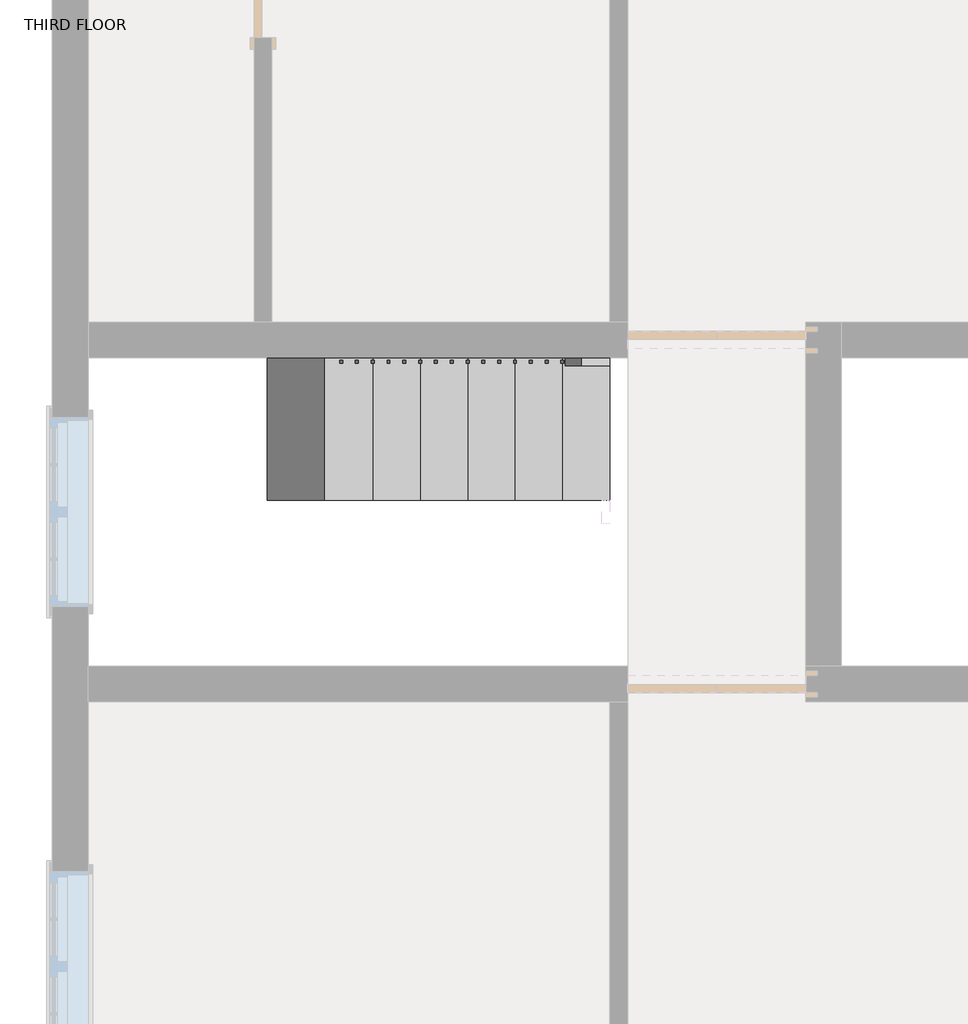
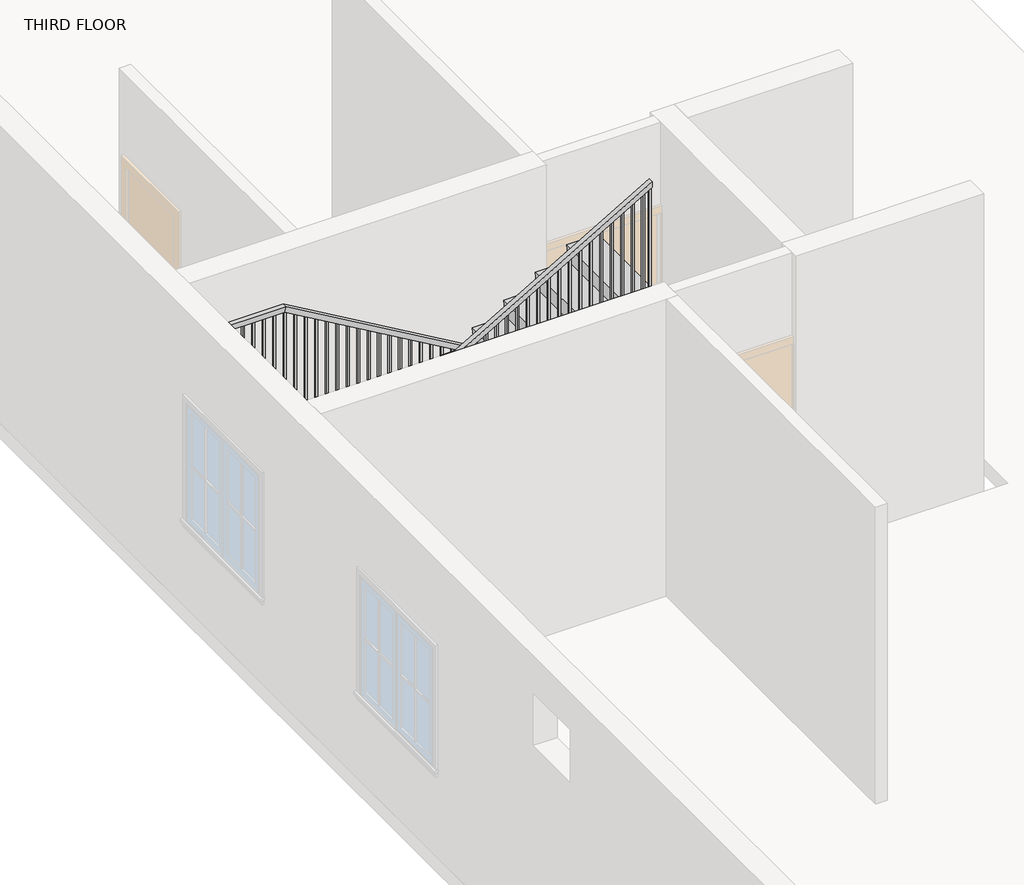
# One storey, part 3 of 4: 1 railing, 1 stair flight.
"""IFC4 building model written with IfcOpenShell, lengths in millimetres."""

from ifc_helpers import new_model, si_unit, frame, origin, place, context, project, spatial, polyline, outline, extrude, faceted_brep, element, save

model = new_model("IFC4")

# Units and contexts
model_context = context("Model", 3, world=origin())
ifc_project = project(units=[si_unit("LENGTHUNIT", "METRE", prefix="MILLI")], contexts=[model_context])

# Site, building, storey
site = spatial("IfcSite", under=ifc_project)
building = spatial("IfcBuilding", under=site)
storey = spatial("IfcBuildingStorey", under=building, Name="THIRD FLOOR", Elevation=9601.2)

# Railing
placement = place(None, origin())
element("IfcRailing", 1, ObjectType="Handrail - Rectangular", at=placement, inside=storey, context=model_context, shape_type="SolidModel", body=[
    faceted_brep([(-2776.8289041, 1499.0153263, 10693.4), (-2776.8289041, 1499.0153263, 10634.5886538), (-2776.8289041, 1549.8153263, 10634.5886538), (-2776.8289041, 1549.8153263, 10693.4), (-5215.2289041, 1499.0153263, 12115.8), (-5228.9626405, 1499.0153263, 12065.0), (-5228.9626405, 1549.8153263, 12065.0), (-5215.2289041, 1549.8153263, 12115.8), (-6078.8289041, 1499.0153263, 12115.8), (-6078.8289041, 1499.0153263, 12065.0), (-6129.6289041, 1549.8153263, 12065.0), (-6129.6289041, 1549.8153263, 12115.8), (-6078.8289041, -380.5846737, 12115.8), (-6078.8289041, -380.5846737, 12065.0), (-6129.6289041, -431.3846737, 12065.0), (-6129.6289041, -431.3846737, 12115.8), (-5520.0289041, -380.5846737, 12115.8), (-5506.2951677, -380.5846737, 12065.0), (-5506.2951677, -431.3846737, 12065.0), (-5520.0289041, -431.3846737, 12115.8), (-2776.8289041, -380.5846737, 13716.0), (-2776.8289041, -431.3846737, 13716.0), (-2776.8289041, -431.3846737, 13657.1886538), (-2776.8289041, -380.5846737, 13657.1886538)], [[[0, 1, 2, 3]], [[1, 0, 4, 5]], [[2, 1, 5, 6]], [[3, 2, 6, 7]], [[0, 3, 7, 4]], [[5, 4, 8, 9]], [[6, 5, 9, 10]], [[7, 6, 10, 11]], [[4, 7, 11, 8]], [[9, 8, 12, 13]], [[10, 9, 13, 14]], [[11, 10, 14, 15]], [[8, 11, 15, 12]], [[13, 12, 16, 17]], [[14, 13, 17, 18]], [[15, 14, 18, 19]], [[12, 15, 19, 16]], [[20, 21, 22, 23]], [[17, 16, 20, 23]], [[18, 17, 23, 22]], [[19, 18, 22, 21]], [[16, 19, 21, 20]]]),
    extrude(outline(polyline([(13618.2949038, -2843.5039041), (13607.1824038, -2862.5539041), (12623.8, -2862.5539041), (12623.8, -2843.5039041), (13618.2949038, -2843.5039041)])), frame((0.0, -415.5096737, 0.0), z_axis=(0.0, 1.0, 0.0), x_axis=(0.0, 0.0, 1.0)), (0.0, 0.0, 1.0), 19.05),
    extrude(outline(polyline([(13559.0282371, -2945.1039041), (13547.9157371, -2964.1539041), (12623.8, -2964.1539041), (12623.8, -2945.1039041), (13559.0282371, -2945.1039041)])), frame((0.0, -415.5096737, 0.0), z_axis=(0.0, 1.0, 0.0), x_axis=(0.0, 0.0, 1.0)), (0.0, 0.0, 1.0), 19.05),
    extrude(outline(polyline([(13499.7615704, -3046.7039041), (13488.6490704, -3065.7539041), (12623.8, -3065.7539041), (12623.8, -3046.7039041), (13499.7615704, -3046.7039041)])), frame((0.0, -415.5096737, 0.0), z_axis=(0.0, 1.0, 0.0), x_axis=(0.0, 0.0, 1.0)), (0.0, 0.0, 1.0), 19.05),
    extrude(outline(polyline([(13440.4949038, -3148.3039041), (13429.3824038, -3167.3539041), (12446.0, -3167.3539041), (12446.0, -3148.3039041), (13440.4949038, -3148.3039041)])), frame((0.0, -415.5096737, 0.0), z_axis=(0.0, 1.0, 0.0), x_axis=(0.0, 0.0, 1.0)), (0.0, 0.0, 1.0), 19.05),
    extrude(outline(polyline([(13381.2282371, -3249.9039041), (13370.1157371, -3268.9539041), (12446.0, -3268.9539041), (12446.0, -3249.9039041), (13381.2282371, -3249.9039041)])), frame((0.0, -415.5096737, 0.0), z_axis=(0.0, 1.0, 0.0), x_axis=(0.0, 0.0, 1.0)), (0.0, 0.0, 1.0), 19.05),
    extrude(outline(polyline([(13321.9615704, -3351.5039041), (13310.8490704, -3370.5539041), (12446.0, -3370.5539041), (12446.0, -3351.5039041), (13321.9615704, -3351.5039041)])), frame((0.0, -415.5096737, 0.0), z_axis=(0.0, 1.0, 0.0), x_axis=(0.0, 0.0, 1.0)), (0.0, 0.0, 1.0), 19.05),
    extrude(outline(polyline([(13262.6949038, -3453.1039041), (13251.5824038, -3472.1539041), (12268.2, -3472.1539041), (12268.2, -3453.1039041), (13262.6949038, -3453.1039041)])), frame((0.0, -415.5096737, 0.0), z_axis=(0.0, 1.0, 0.0), x_axis=(0.0, 0.0, 1.0)), (0.0, 0.0, 1.0), 19.05),
    extrude(outline(polyline([(13203.4282371, -3554.7039041), (13192.3157371, -3573.7539041), (12268.2, -3573.7539041), (12268.2, -3554.7039041), (13203.4282371, -3554.7039041)])), frame((0.0, -415.5096737, 0.0), z_axis=(0.0, 1.0, 0.0), x_axis=(0.0, 0.0, 1.0)), (0.0, 0.0, 1.0), 19.05),
    extrude(outline(polyline([(13144.1615704, -3656.3039041), (13133.0490704, -3675.3539041), (12268.2, -3675.3539041), (12268.2, -3656.3039041), (13144.1615704, -3656.3039041)])), frame((0.0, -415.5096737, 0.0), z_axis=(0.0, 1.0, 0.0), x_axis=(0.0, 0.0, 1.0)), (0.0, 0.0, 1.0), 19.05),
    extrude(outline(polyline([(13084.8949038, -3757.9039041), (13073.7824038, -3776.9539041), (12090.4, -3776.9539041), (12090.4, -3757.9039041), (13084.8949038, -3757.9039041)])), frame((0.0, -415.5096737, 0.0), z_axis=(0.0, 1.0, 0.0), x_axis=(0.0, 0.0, 1.0)), (0.0, 0.0, 1.0), 19.05),
    extrude(outline(polyline([(13025.6282371, -3859.5039041), (13014.5157371, -3878.5539041), (12090.4, -3878.5539041), (12090.4, -3859.5039041), (13025.6282371, -3859.5039041)])), frame((0.0, -415.5096737, 0.0), z_axis=(0.0, 1.0, 0.0), x_axis=(0.0, 0.0, 1.0)), (0.0, 0.0, 1.0), 19.05),
    extrude(outline(polyline([(12966.3615704, -3961.1039041), (12955.2490704, -3980.1539041), (12090.4, -3980.1539041), (12090.4, -3961.1039041), (12966.3615704, -3961.1039041)])), frame((0.0, -415.5096737, 0.0), z_axis=(0.0, 1.0, 0.0), x_axis=(0.0, 0.0, 1.0)), (0.0, 0.0, 1.0), 19.05),
    extrude(outline(polyline([(12907.0949038, -4062.7039041), (12895.9824038, -4081.7539041), (11912.6, -4081.7539041), (11912.6, -4062.7039041), (12907.0949038, -4062.7039041)])), frame((0.0, -415.5096737, 0.0), z_axis=(0.0, 1.0, 0.0), x_axis=(0.0, 0.0, 1.0)), (0.0, 0.0, 1.0), 19.05),
    extrude(outline(polyline([(12847.8282371, -4164.3039041), (12836.7157371, -4183.3539041), (11912.6, -4183.3539041), (11912.6, -4164.3039041), (12847.8282371, -4164.3039041)])), frame((0.0, -415.5096737, 0.0), z_axis=(0.0, 1.0, 0.0), x_axis=(0.0, 0.0, 1.0)), (0.0, 0.0, 1.0), 19.05),
    extrude(outline(polyline([(12788.5615704, -4265.9039041), (12777.4490704, -4284.9539041), (11912.6, -4284.9539041), (11912.6, -4265.9039041), (12788.5615704, -4265.9039041)])), frame((0.0, -415.5096737, 0.0), z_axis=(0.0, 1.0, 0.0), x_axis=(0.0, 0.0, 1.0)), (0.0, 0.0, 1.0), 19.05),
    extrude(outline(polyline([(12729.2949038, -4367.5039041), (12718.1824038, -4386.5539041), (11734.8, -4386.5539041), (11734.8, -4367.5039041), (12729.2949038, -4367.5039041)])), frame((0.0, -415.5096737, 0.0), z_axis=(0.0, 1.0, 0.0), x_axis=(0.0, 0.0, 1.0)), (0.0, 0.0, 1.0), 19.05),
    extrude(outline(polyline([(12670.0282371, -4469.1039041), (12658.9157371, -4488.1539041), (11734.8, -4488.1539041), (11734.8, -4469.1039041), (12670.0282371, -4469.1039041)])), frame((0.0, -415.5096737, 0.0), z_axis=(0.0, 1.0, 0.0), x_axis=(0.0, 0.0, 1.0)), (0.0, 0.0, 1.0), 19.05),
    extrude(outline(polyline([(12610.7615704, -4570.7039041), (12599.6490704, -4589.7539041), (11734.8, -4589.7539041), (11734.8, -4570.7039041), (12610.7615704, -4570.7039041)])), frame((0.0, -415.5096737, 0.0), z_axis=(0.0, 1.0, 0.0), x_axis=(0.0, 0.0, 1.0)), (0.0, 0.0, 1.0), 19.05),
    extrude(outline(polyline([(12551.4949038, -4672.3039041), (12540.3824038, -4691.3539041), (11557.0, -4691.3539041), (11557.0, -4672.3039041), (12551.4949038, -4672.3039041)])), frame((0.0, -415.5096737, 0.0), z_axis=(0.0, 1.0, 0.0), x_axis=(0.0, 0.0, 1.0)), (0.0, 0.0, 1.0), 19.05),
    extrude(outline(polyline([(12492.2282371, -4773.9039041), (12481.1157371, -4792.9539041), (11557.0, -4792.9539041), (11557.0, -4773.9039041), (12492.2282371, -4773.9039041)])), frame((0.0, -415.5096737, 0.0), z_axis=(0.0, 1.0, 0.0), x_axis=(0.0, 0.0, 1.0)), (0.0, 0.0, 1.0), 19.05),
    extrude(outline(polyline([(12432.9615704, -4875.5039041), (12421.8490704, -4894.5539041), (11557.0, -4894.5539041), (11557.0, -4875.5039041), (12432.9615704, -4875.5039041)])), frame((0.0, -415.5096737, 0.0), z_axis=(0.0, 1.0, 0.0), x_axis=(0.0, 0.0, 1.0)), (0.0, 0.0, 1.0), 19.05),
    extrude(outline(polyline([(12373.6949038, -4977.1039041), (12362.5824038, -4996.1539041), (11379.2, -4996.1539041), (11379.2, -4977.1039041), (12373.6949038, -4977.1039041)])), frame((0.0, -415.5096737, 0.0), z_axis=(0.0, 1.0, 0.0), x_axis=(0.0, 0.0, 1.0)), (0.0, 0.0, 1.0), 19.05),
    extrude(outline(polyline([(12314.4282371, -5078.7039041), (12303.3157371, -5097.7539041), (11379.2, -5097.7539041), (11379.2, -5078.7039041), (12314.4282371, -5078.7039041)])), frame((0.0, -415.5096737, 0.0), z_axis=(0.0, 1.0, 0.0), x_axis=(0.0, 0.0, 1.0)), (0.0, 0.0, 1.0), 19.05),
    extrude(outline(polyline([(12255.1615704, -5180.3039041), (12244.0490704, -5199.3539041), (11379.2, -5199.3539041), (11379.2, -5180.3039041), (12255.1615704, -5180.3039041)])), frame((0.0, -415.5096737, 0.0), z_axis=(0.0, 1.0, 0.0), x_axis=(0.0, 0.0, 1.0)), (0.0, 0.0, 1.0), 19.05),
    extrude(outline(polyline([(12195.8949038, -5281.9039041), (12184.7824038, -5300.9539041), (11201.4, -5300.9539041), (11201.4, -5281.9039041), (12195.8949038, -5281.9039041)])), frame((0.0, -415.5096737, 0.0), z_axis=(0.0, 1.0, 0.0), x_axis=(0.0, 0.0, 1.0)), (0.0, 0.0, 1.0), 19.05),
    extrude(outline(polyline([(12136.6282371, -5383.5039041), (12125.5157371, -5402.5539041), (11201.4, -5402.5539041), (11201.4, -5383.5039041), (12136.6282371, -5383.5039041)])), frame((0.0, -415.5096737, 0.0), z_axis=(0.0, 1.0, 0.0), x_axis=(0.0, 0.0, 1.0)), (0.0, 0.0, 1.0), 19.05),
    extrude(outline(polyline([(12077.3615704, -5485.1039041), (12066.2490704, -5504.1539041), (11201.4, -5504.1539041), (11201.4, -5485.1039041), (12077.3615704, -5485.1039041)])), frame((0.0, -415.5096737, 0.0), z_axis=(0.0, 1.0, 0.0), x_axis=(0.0, 0.0, 1.0)), (0.0, 0.0, 1.0), 19.05),
    extrude(outline(polyline([(-5605.7539041, -415.5096737), (-5605.7539041, -396.4596737), (-5586.7039041, -396.4596737), (-5586.7039041, -415.5096737), (-5605.7539041, -415.5096737)])), frame((0.0, 0.0, 11201.4), z_axis=(0.0, 0.0, 1.0), x_axis=(1.0, 0.0, 0.0)), (0.0, 0.0, 1.0), 863.6),
    extrude(outline(polyline([(-5707.3539041, -415.5096737), (-5707.3539041, -396.4596737), (-5688.3039041, -396.4596737), (-5688.3039041, -415.5096737), (-5707.3539041, -415.5096737)])), frame((0.0, 0.0, 11201.4), z_axis=(0.0, 0.0, 1.0), x_axis=(1.0, 0.0, 0.0)), (0.0, 0.0, 1.0), 863.6),
    extrude(outline(polyline([(-5808.9539041, -415.5096737), (-5808.9539041, -396.4596737), (-5789.9039041, -396.4596737), (-5789.9039041, -415.5096737), (-5808.9539041, -415.5096737)])), frame((0.0, 0.0, 11201.4), z_axis=(0.0, 0.0, 1.0), x_axis=(1.0, 0.0, 0.0)), (0.0, 0.0, 1.0), 863.6),
    extrude(outline(polyline([(-5910.5539041, -415.5096737), (-5910.5539041, -396.4596737), (-5891.5039041, -396.4596737), (-5891.5039041, -415.5096737), (-5910.5539041, -415.5096737)])), frame((0.0, 0.0, 11201.4), z_axis=(0.0, 0.0, 1.0), x_axis=(1.0, 0.0, 0.0)), (0.0, 0.0, 1.0), 863.6),
    extrude(outline(polyline([(-6012.1539041, -415.5096737), (-6012.1539041, -396.4596737), (-5993.1039041, -396.4596737), (-5993.1039041, -415.5096737), (-6012.1539041, -415.5096737)])), frame((0.0, 0.0, 11201.4), z_axis=(0.0, 0.0, 1.0), x_axis=(1.0, 0.0, 0.0)), (0.0, 0.0, 1.0), 863.6),
    extrude(outline(polyline([(-6113.7539041, -294.8596737), (-6094.7039041, -294.8596737), (-6094.7039041, -313.9096737), (-6113.7539041, -313.9096737), (-6113.7539041, -294.8596737)])), frame((0.0, 0.0, 11201.4), z_axis=(0.0, 0.0, 1.0), x_axis=(1.0, 0.0, 0.0)), (0.0, 0.0, 1.0), 863.6),
    extrude(outline(polyline([(-6113.7539041, -193.2596737), (-6094.7039041, -193.2596737), (-6094.7039041, -212.3096737), (-6113.7539041, -212.3096737), (-6113.7539041, -193.2596737)])), frame((0.0, 0.0, 11201.4), z_axis=(0.0, 0.0, 1.0), x_axis=(1.0, 0.0, 0.0)), (0.0, 0.0, 1.0), 863.6),
    extrude(outline(polyline([(-6113.7539041, -91.6596737), (-6094.7039041, -91.6596737), (-6094.7039041, -110.7096737), (-6113.7539041, -110.7096737), (-6113.7539041, -91.6596737)])), frame((0.0, 0.0, 11201.4), z_axis=(0.0, 0.0, 1.0), x_axis=(1.0, 0.0, 0.0)), (0.0, 0.0, 1.0), 863.6),
    extrude(outline(polyline([(-6113.7539041, 9.9403263), (-6094.7039041, 9.9403263), (-6094.7039041, -9.1096737), (-6113.7539041, -9.1096737), (-6113.7539041, 9.9403263)])), frame((0.0, 0.0, 11201.4), z_axis=(0.0, 0.0, 1.0), x_axis=(1.0, 0.0, 0.0)), (0.0, 0.0, 1.0), 863.6),
    extrude(outline(polyline([(-6113.7539041, 111.5403263), (-6094.7039041, 111.5403263), (-6094.7039041, 92.4903263), (-6113.7539041, 92.4903263), (-6113.7539041, 111.5403263)])), frame((0.0, 0.0, 11201.4), z_axis=(0.0, 0.0, 1.0), x_axis=(1.0, 0.0, 0.0)), (0.0, 0.0, 1.0), 863.6),
    extrude(outline(polyline([(-6113.7539041, 213.1403263), (-6094.7039041, 213.1403263), (-6094.7039041, 194.0903263), (-6113.7539041, 194.0903263), (-6113.7539041, 213.1403263)])), frame((0.0, 0.0, 11201.4), z_axis=(0.0, 0.0, 1.0), x_axis=(1.0, 0.0, 0.0)), (0.0, 0.0, 1.0), 863.6),
    extrude(outline(polyline([(-6113.7539041, 314.7403263), (-6094.7039041, 314.7403263), (-6094.7039041, 295.6903263), (-6113.7539041, 295.6903263), (-6113.7539041, 314.7403263)])), frame((0.0, 0.0, 11201.4), z_axis=(0.0, 0.0, 1.0), x_axis=(1.0, 0.0, 0.0)), (0.0, 0.0, 1.0), 863.6),
    extrude(outline(polyline([(-6113.7539041, 416.3403263), (-6094.7039041, 416.3403263), (-6094.7039041, 397.2903263), (-6113.7539041, 397.2903263), (-6113.7539041, 416.3403263)])), frame((0.0, 0.0, 11201.4), z_axis=(0.0, 0.0, 1.0), x_axis=(1.0, 0.0, 0.0)), (0.0, 0.0, 1.0), 863.6),
    extrude(outline(polyline([(-6113.7539041, 517.9403263), (-6094.7039041, 517.9403263), (-6094.7039041, 498.8903263), (-6113.7539041, 498.8903263), (-6113.7539041, 517.9403263)])), frame((0.0, 0.0, 11201.4), z_axis=(0.0, 0.0, 1.0), x_axis=(1.0, 0.0, 0.0)), (0.0, 0.0, 1.0), 863.6),
    extrude(outline(polyline([(-6113.7539041, 619.5403263), (-6094.7039041, 619.5403263), (-6094.7039041, 600.4903263), (-6113.7539041, 600.4903263), (-6113.7539041, 619.5403263)])), frame((0.0, 0.0, 11201.4), z_axis=(0.0, 0.0, 1.0), x_axis=(1.0, 0.0, 0.0)), (0.0, 0.0, 1.0), 863.6),
    extrude(outline(polyline([(-6113.7539041, 721.1403263), (-6094.7039041, 721.1403263), (-6094.7039041, 702.0903263), (-6113.7539041, 702.0903263), (-6113.7539041, 721.1403263)])), frame((0.0, 0.0, 11201.4), z_axis=(0.0, 0.0, 1.0), x_axis=(1.0, 0.0, 0.0)), (0.0, 0.0, 1.0), 863.6),
    extrude(outline(polyline([(-6113.7539041, 822.7403263), (-6094.7039041, 822.7403263), (-6094.7039041, 803.6903263), (-6113.7539041, 803.6903263), (-6113.7539041, 822.7403263)])), frame((0.0, 0.0, 11201.4), z_axis=(0.0, 0.0, 1.0), x_axis=(1.0, 0.0, 0.0)), (0.0, 0.0, 1.0), 863.6),
    extrude(outline(polyline([(-6113.7539041, 924.3403263), (-6094.7039041, 924.3403263), (-6094.7039041, 905.2903263), (-6113.7539041, 905.2903263), (-6113.7539041, 924.3403263)])), frame((0.0, 0.0, 11201.4), z_axis=(0.0, 0.0, 1.0), x_axis=(1.0, 0.0, 0.0)), (0.0, 0.0, 1.0), 863.6),
    extrude(outline(polyline([(-6113.7539041, 1025.9403263), (-6094.7039041, 1025.9403263), (-6094.7039041, 1006.8903263), (-6113.7539041, 1006.8903263), (-6113.7539041, 1025.9403263)])), frame((0.0, 0.0, 11201.4), z_axis=(0.0, 0.0, 1.0), x_axis=(1.0, 0.0, 0.0)), (0.0, 0.0, 1.0), 863.6),
    extrude(outline(polyline([(-6113.7539041, 1127.5403263), (-6094.7039041, 1127.5403263), (-6094.7039041, 1108.4903263), (-6113.7539041, 1108.4903263), (-6113.7539041, 1127.5403263)])), frame((0.0, 0.0, 11201.4), z_axis=(0.0, 0.0, 1.0), x_axis=(1.0, 0.0, 0.0)), (0.0, 0.0, 1.0), 863.6),
    extrude(outline(polyline([(-6113.7539041, 1229.1403263), (-6094.7039041, 1229.1403263), (-6094.7039041, 1210.0903263), (-6113.7539041, 1210.0903263), (-6113.7539041, 1229.1403263)])), frame((0.0, 0.0, 11201.4), z_axis=(0.0, 0.0, 1.0), x_axis=(1.0, 0.0, 0.0)), (0.0, 0.0, 1.0), 863.6),
    extrude(outline(polyline([(-6113.7539041, 1330.7403263), (-6094.7039041, 1330.7403263), (-6094.7039041, 1311.6903263), (-6113.7539041, 1311.6903263), (-6113.7539041, 1330.7403263)])), frame((0.0, 0.0, 11201.4), z_axis=(0.0, 0.0, 1.0), x_axis=(1.0, 0.0, 0.0)), (0.0, 0.0, 1.0), 863.6),
    extrude(outline(polyline([(-6113.7539041, 1432.3403263), (-6094.7039041, 1432.3403263), (-6094.7039041, 1413.2903263), (-6113.7539041, 1413.2903263), (-6113.7539041, 1432.3403263)])), frame((0.0, 0.0, 11201.4), z_axis=(0.0, 0.0, 1.0), x_axis=(1.0, 0.0, 0.0)), (0.0, 0.0, 1.0), 863.6),
    extrude(outline(polyline([(-6018.5039041, 1533.9403263), (-6018.5039041, 1514.8903263), (-6037.5539041, 1514.8903263), (-6037.5539041, 1533.9403263), (-6018.5039041, 1533.9403263)])), frame((0.0, 0.0, 11201.4), z_axis=(0.0, 0.0, 1.0), x_axis=(1.0, 0.0, 0.0)), (0.0, 0.0, 1.0), 863.6),
    extrude(outline(polyline([(-5916.9039041, 1533.9403263), (-5916.9039041, 1514.8903263), (-5935.9539041, 1514.8903263), (-5935.9539041, 1533.9403263), (-5916.9039041, 1533.9403263)])), frame((0.0, 0.0, 11201.4), z_axis=(0.0, 0.0, 1.0), x_axis=(1.0, 0.0, 0.0)), (0.0, 0.0, 1.0), 863.6),
    extrude(outline(polyline([(-5815.3039041, 1533.9403263), (-5815.3039041, 1514.8903263), (-5834.3539041, 1514.8903263), (-5834.3539041, 1533.9403263), (-5815.3039041, 1533.9403263)])), frame((0.0, 0.0, 11201.4), z_axis=(0.0, 0.0, 1.0), x_axis=(1.0, 0.0, 0.0)), (0.0, 0.0, 1.0), 863.6),
    extrude(outline(polyline([(-5713.7039041, 1533.9403263), (-5713.7039041, 1514.8903263), (-5732.7539041, 1514.8903263), (-5732.7539041, 1533.9403263), (-5713.7039041, 1533.9403263)])), frame((0.0, 0.0, 11201.4), z_axis=(0.0, 0.0, 1.0), x_axis=(1.0, 0.0, 0.0)), (0.0, 0.0, 1.0), 863.6),
    extrude(outline(polyline([(-5612.1039041, 1533.9403263), (-5612.1039041, 1514.8903263), (-5631.1539041, 1514.8903263), (-5631.1539041, 1533.9403263), (-5612.1039041, 1533.9403263)])), frame((0.0, 0.0, 11201.4), z_axis=(0.0, 0.0, 1.0), x_axis=(1.0, 0.0, 0.0)), (0.0, 0.0, 1.0), 863.6),
    extrude(outline(polyline([(-5510.5039041, 1533.9403263), (-5510.5039041, 1514.8903263), (-5529.5539041, 1514.8903263), (-5529.5539041, 1533.9403263), (-5510.5039041, 1533.9403263)])), frame((0.0, 0.0, 11201.4), z_axis=(0.0, 0.0, 1.0), x_axis=(1.0, 0.0, 0.0)), (0.0, 0.0, 1.0), 863.6),
    extrude(outline(polyline([(-5408.9039041, 1533.9403263), (-5408.9039041, 1514.8903263), (-5427.9539041, 1514.8903263), (-5427.9539041, 1533.9403263), (-5408.9039041, 1533.9403263)])), frame((0.0, 0.0, 11201.4), z_axis=(0.0, 0.0, 1.0), x_axis=(1.0, 0.0, 0.0)), (0.0, 0.0, 1.0), 863.6),
    extrude(outline(polyline([(-5307.3039041, 1533.9403263), (-5307.3039041, 1514.8903263), (-5326.3539041, 1514.8903263), (-5326.3539041, 1533.9403263), (-5307.3039041, 1533.9403263)])), frame((0.0, 0.0, 11201.4), z_axis=(0.0, 0.0, 1.0), x_axis=(1.0, 0.0, 0.0)), (0.0, 0.0, 1.0), 863.6),
    extrude(outline(polyline([(12051.4324038, -5205.7039041), (12062.5449038, -5224.7539041), (11201.4, -5224.7539041), (11201.4, -5205.7039041), (12051.4324038, -5205.7039041)])), frame((0.0, 1514.8903263, 0.0), z_axis=(0.0, 1.0, 0.0), x_axis=(0.0, 0.0, 1.0)), (0.0, 0.0, 1.0), 19.05),
    extrude(outline(polyline([(11992.1657371, -5104.1039041), (12003.2782371, -5123.1539041), (11023.6, -5123.1539041), (11023.6, -5104.1039041), (11992.1657371, -5104.1039041)])), frame((0.0, 1514.8903263, 0.0), z_axis=(0.0, 1.0, 0.0), x_axis=(0.0, 0.0, 1.0)), (0.0, 0.0, 1.0), 19.05),
    extrude(outline(polyline([(11932.8990704, -5002.5039041), (11944.0115704, -5021.5539041), (11023.6, -5021.5539041), (11023.6, -5002.5039041), (11932.8990704, -5002.5039041)])), frame((0.0, 1514.8903263, 0.0), z_axis=(0.0, 1.0, 0.0), x_axis=(0.0, 0.0, 1.0)), (0.0, 0.0, 1.0), 19.05),
    extrude(outline(polyline([(11873.6324038, -4900.9039041), (11884.7449038, -4919.9539041), (11023.6, -4919.9539041), (11023.6, -4900.9039041), (11873.6324038, -4900.9039041)])), frame((0.0, 1514.8903263, 0.0), z_axis=(0.0, 1.0, 0.0), x_axis=(0.0, 0.0, 1.0)), (0.0, 0.0, 1.0), 19.05),
    extrude(outline(polyline([(11814.3657371, -4799.3039041), (11825.4782371, -4818.3539041), (10845.8, -4818.3539041), (10845.8, -4799.3039041), (11814.3657371, -4799.3039041)])), frame((0.0, 1514.8903263, 0.0), z_axis=(0.0, 1.0, 0.0), x_axis=(0.0, 0.0, 1.0)), (0.0, 0.0, 1.0), 19.05),
    extrude(outline(polyline([(11755.0990704, -4697.7039041), (11766.2115704, -4716.7539041), (10845.8, -4716.7539041), (10845.8, -4697.7039041), (11755.0990704, -4697.7039041)])), frame((0.0, 1514.8903263, 0.0), z_axis=(0.0, 1.0, 0.0), x_axis=(0.0, 0.0, 1.0)), (0.0, 0.0, 1.0), 19.05),
    extrude(outline(polyline([(11695.8324038, -4596.1039041), (11706.9449038, -4615.1539041), (10845.8, -4615.1539041), (10845.8, -4596.1039041), (11695.8324038, -4596.1039041)])), frame((0.0, 1514.8903263, 0.0), z_axis=(0.0, 1.0, 0.0), x_axis=(0.0, 0.0, 1.0)), (0.0, 0.0, 1.0), 19.05),
    extrude(outline(polyline([(11636.5657371, -4494.5039041), (11647.6782371, -4513.5539041), (10668.0, -4513.5539041), (10668.0, -4494.5039041), (11636.5657371, -4494.5039041)])), frame((0.0, 1514.8903263, 0.0), z_axis=(0.0, 1.0, 0.0), x_axis=(0.0, 0.0, 1.0)), (0.0, 0.0, 1.0), 19.05),
    extrude(outline(polyline([(11577.2990704, -4392.9039041), (11588.4115704, -4411.9539041), (10668.0, -4411.9539041), (10668.0, -4392.9039041), (11577.2990704, -4392.9039041)])), frame((0.0, 1514.8903263, 0.0), z_axis=(0.0, 1.0, 0.0), x_axis=(0.0, 0.0, 1.0)), (0.0, 0.0, 1.0), 19.05),
    extrude(outline(polyline([(11518.0324038, -4291.3039041), (11529.1449038, -4310.3539041), (10668.0, -4310.3539041), (10668.0, -4291.3039041), (11518.0324038, -4291.3039041)])), frame((0.0, 1514.8903263, 0.0), z_axis=(0.0, 1.0, 0.0), x_axis=(0.0, 0.0, 1.0)), (0.0, 0.0, 1.0), 19.05),
    extrude(outline(polyline([(11458.7657371, -4189.7039041), (11469.8782371, -4208.7539041), (10490.2, -4208.7539041), (10490.2, -4189.7039041), (11458.7657371, -4189.7039041)])), frame((0.0, 1514.8903263, 0.0), z_axis=(0.0, 1.0, 0.0), x_axis=(0.0, 0.0, 1.0)), (0.0, 0.0, 1.0), 19.05),
    extrude(outline(polyline([(11399.4990704, -4088.1039041), (11410.6115704, -4107.1539041), (10490.2, -4107.1539041), (10490.2, -4088.1039041), (11399.4990704, -4088.1039041)])), frame((0.0, 1514.8903263, 0.0), z_axis=(0.0, 1.0, 0.0), x_axis=(0.0, 0.0, 1.0)), (0.0, 0.0, 1.0), 19.05),
    extrude(outline(polyline([(11340.2324038, -3986.5039041), (11351.3449038, -4005.5539041), (10490.2, -4005.5539041), (10490.2, -3986.5039041), (11340.2324038, -3986.5039041)])), frame((0.0, 1514.8903263, 0.0), z_axis=(0.0, 1.0, 0.0), x_axis=(0.0, 0.0, 1.0)), (0.0, 0.0, 1.0), 19.05),
    extrude(outline(polyline([(11280.9657371, -3884.9039041), (11292.0782371, -3903.9539041), (10312.4, -3903.9539041), (10312.4, -3884.9039041), (11280.9657371, -3884.9039041)])), frame((0.0, 1514.8903263, 0.0), z_axis=(0.0, 1.0, 0.0), x_axis=(0.0, 0.0, 1.0)), (0.0, 0.0, 1.0), 19.05),
    extrude(outline(polyline([(11221.6990704, -3783.3039041), (11232.8115704, -3802.3539041), (10312.4, -3802.3539041), (10312.4, -3783.3039041), (11221.6990704, -3783.3039041)])), frame((0.0, 1514.8903263, 0.0), z_axis=(0.0, 1.0, 0.0), x_axis=(0.0, 0.0, 1.0)), (0.0, 0.0, 1.0), 19.05),
    extrude(outline(polyline([(11162.4324038, -3681.7039041), (11173.5449038, -3700.7539041), (10312.4, -3700.7539041), (10312.4, -3681.7039041), (11162.4324038, -3681.7039041)])), frame((0.0, 1514.8903263, 0.0), z_axis=(0.0, 1.0, 0.0), x_axis=(0.0, 0.0, 1.0)), (0.0, 0.0, 1.0), 19.05),
    extrude(outline(polyline([(11103.1657371, -3580.1039041), (11114.2782371, -3599.1539041), (10134.6, -3599.1539041), (10134.6, -3580.1039041), (11103.1657371, -3580.1039041)])), frame((0.0, 1514.8903263, 0.0), z_axis=(0.0, 1.0, 0.0), x_axis=(0.0, 0.0, 1.0)), (0.0, 0.0, 1.0), 19.05),
    extrude(outline(polyline([(11043.8990704, -3478.5039041), (11055.0115704, -3497.5539041), (10134.6, -3497.5539041), (10134.6, -3478.5039041), (11043.8990704, -3478.5039041)])), frame((0.0, 1514.8903263, 0.0), z_axis=(0.0, 1.0, 0.0), x_axis=(0.0, 0.0, 1.0)), (0.0, 0.0, 1.0), 19.05),
    extrude(outline(polyline([(10984.6324038, -3376.9039041), (10995.7449038, -3395.9539041), (10134.6, -3395.9539041), (10134.6, -3376.9039041), (10984.6324038, -3376.9039041)])), frame((0.0, 1514.8903263, 0.0), z_axis=(0.0, 1.0, 0.0), x_axis=(0.0, 0.0, 1.0)), (0.0, 0.0, 1.0), 19.05),
    extrude(outline(polyline([(10925.3657371, -3275.3039041), (10936.4782371, -3294.3539041), (9956.8, -3294.3539041), (9956.8, -3275.3039041), (10925.3657371, -3275.3039041)])), frame((0.0, 1514.8903263, 0.0), z_axis=(0.0, 1.0, 0.0), x_axis=(0.0, 0.0, 1.0)), (0.0, 0.0, 1.0), 19.05),
    extrude(outline(polyline([(10866.0990704, -3173.7039041), (10877.2115704, -3192.7539041), (9956.8, -3192.7539041), (9956.8, -3173.7039041), (10866.0990704, -3173.7039041)])), frame((0.0, 1514.8903263, 0.0), z_axis=(0.0, 1.0, 0.0), x_axis=(0.0, 0.0, 1.0)), (0.0, 0.0, 1.0), 19.05),
    extrude(outline(polyline([(10806.8324038, -3072.1039041), (10817.9449038, -3091.1539041), (9956.8, -3091.1539041), (9956.8, -3072.1039041), (10806.8324038, -3072.1039041)])), frame((0.0, 1514.8903263, 0.0), z_axis=(0.0, 1.0, 0.0), x_axis=(0.0, 0.0, 1.0)), (0.0, 0.0, 1.0), 19.05),
    extrude(outline(polyline([(10747.5657371, -2970.5039041), (10758.6782371, -2989.5539041), (9779.0, -2989.5539041), (9779.0, -2970.5039041), (10747.5657371, -2970.5039041)])), frame((0.0, 1514.8903263, 0.0), z_axis=(0.0, 1.0, 0.0), x_axis=(0.0, 0.0, 1.0)), (0.0, 0.0, 1.0), 19.05),
    extrude(outline(polyline([(10688.2990704, -2868.9039041), (10699.4115704, -2887.9539041), (9779.0, -2887.9539041), (9779.0, -2868.9039041), (10688.2990704, -2868.9039041)])), frame((0.0, 1514.8903263, 0.0), z_axis=(0.0, 1.0, 0.0), x_axis=(0.0, 0.0, 1.0)), (0.0, 0.0, 1.0), 19.05),
    extrude(outline(polyline([(-6113.7539041, -396.4596737), (-6094.7039041, -396.4596737), (-6094.7039041, -415.5096737), (-6113.7539041, -415.5096737), (-6113.7539041, -396.4596737)])), frame((0.0, 0.0, 11201.4), z_axis=(0.0, 0.0, 1.0), x_axis=(1.0, 0.0, 0.0)), (0.0, 0.0, 1.0), 863.6),
    extrude(outline(polyline([(-6094.7039041, 1533.9403263), (-6094.7039041, 1514.8903263), (-6113.7539041, 1514.8903263), (-6113.7539041, 1533.9403263), (-6094.7039041, 1533.9403263)])), frame((0.0, 0.0, 11201.4), z_axis=(0.0, 0.0, 1.0), x_axis=(1.0, 0.0, 0.0)), (0.0, 0.0, 1.0), 863.6),
    extrude(outline(polyline([(13657.1886538, -2776.8289041), (13646.0761538, -2795.8789041), (12623.8, -2795.8789041), (12623.8, -2776.8289041), (13657.1886538, -2776.8289041)])), frame((0.0, -415.5096737, 0.0), z_axis=(0.0, 1.0, 0.0), x_axis=(0.0, 0.0, 1.0)), (0.0, 0.0, 1.0), 19.05),
    extrude(outline(polyline([(10634.5886538, -2776.8289041), (10645.7011538, -2795.8789041), (9779.0, -2795.8789041), (9779.0, -2776.8289041), (10634.5886538, -2776.8289041)])), frame((0.0, 1514.8903263, 0.0), z_axis=(0.0, 1.0, 0.0), x_axis=(0.0, 0.0, 1.0)), (0.0, 0.0, 1.0), 19.05),
])

# Stair flight
element("IfcStairFlight", 2, ObjectType="3/4\" Nosing", at=placement, inside=storey, context=model_context, shape_type="Brep", body=[
    faceted_brep([(-2776.8289041, 635.4153263, 9779.0), (-2776.8289041, 1549.8153263, 9779.0), (-3100.6789041, 1549.8153263, 9779.0), (-3100.6789041, 635.4153263, 9779.0), (-3100.6789041, 635.4153263, 9705.4858172), (-2921.9032174, 635.4153263, 9601.2), (-2795.8789041, 635.4153263, 9601.2), (-2795.8789041, 1549.8153263, 9601.2), (-2921.9032174, 1549.8153263, 9601.2), (-3100.6789041, 1549.8153263, 9705.4858172), (-3081.6289041, 635.4153263, 9956.8), (-3081.6289041, 1549.8153263, 9956.8), (-3405.4789041, 1549.8153263, 9956.8), (-3405.4789041, 635.4153263, 9956.8), (-3405.4789041, 635.4153263, 9883.2858172), (-3405.4789041, 1549.8153263, 9883.2858172), (-3386.4289041, 635.4153263, 10134.6), (-3386.4289041, 1549.8153263, 10134.6), (-3710.2789041, 1549.8153263, 10134.6), (-3710.2789041, 635.4153263, 10134.6), (-3710.2789041, 635.4153263, 10061.0858172), (-3710.2789041, 1549.8153263, 10061.0858172), (-3691.2289041, 635.4153263, 10312.4), (-3691.2289041, 1549.8153263, 10312.4), (-4015.0789041, 1549.8153263, 10312.4), (-4015.0789041, 635.4153263, 10312.4), (-4015.0789041, 635.4153263, 10238.8858172), (-4015.0789041, 1549.8153263, 10238.8858172), (-3996.0289041, 635.4153263, 10490.2), (-3996.0289041, 1549.8153263, 10490.2), (-4319.8789041, 1549.8153263, 10490.2), (-4319.8789041, 635.4153263, 10490.2), (-4300.8289041, 635.4153263, 10668.0), (-4624.6789041, 635.4153263, 10668.0), (-4605.6289041, 635.4153263, 10845.8), (-4929.4789041, 635.4153263, 10845.8), (-4910.4289041, 635.4153263, 11023.6), (-5234.2789041, 635.4153263, 11023.6), (-5222.0324755, 635.4153263, 11137.9), (-5556.2460745, 635.4153263, 11137.9), (-4319.8789041, 1549.8153263, 10416.6858172), (-4300.8289041, 1549.8153263, 10668.0), (-4624.6789041, 1549.8153263, 10668.0), (-4624.6789041, 1549.8153263, 10594.4858172), (-4605.6289041, 1549.8153263, 10845.8), (-4929.4789041, 1549.8153263, 10845.8), (-4929.4789041, 1549.8153263, 10772.2858172), (-4910.4289041, 1549.8153263, 11023.6), (-5234.2789041, 1549.8153263, 11023.6), (-5234.2789041, 1549.8153263, 10950.0858172), (-5070.1545907, 483.0153263, 11201.4), (-2776.8289041, 483.0153263, 11201.4), (-2776.8289041, 635.4153263, 11201.4), (-3836.3032174, 635.4153263, 11201.4), (-5215.2289041, 635.4153263, 11201.4), (-5215.2289041, 1549.8153263, 11201.4), (-5556.2460745, 1549.8153263, 11201.4), (-6129.6289041, 1549.8153263, 11201.4), (-6129.6289041, -431.3846737, 11201.4), (-5196.1789041, -431.3846737, 11201.4), (-5196.1789041, 483.0153263, 11201.4), (-5179.0117336, 483.0153263, 11137.9), (-2776.8289041, 483.0153263, 11137.9), (-2776.8289041, 635.4153263, 11137.9), (-3727.4460745, 635.4153263, 11137.9), (-5556.2460745, 1549.8153263, 11137.9), (-6129.6289041, 1549.8153263, 11137.9), (-6129.6289041, -431.3846737, 11137.9), (-5196.1789041, -431.3846737, 11137.9), (-5215.2289041, 483.0153263, 11379.2), (-5215.2289041, -431.3846737, 11379.2), (-5179.0117336, -431.3846737, 11379.2), (-4891.3789041, -431.3846737, 11379.2), (-4891.3789041, 483.0153263, 11379.2), (-4891.3789041, 483.0153263, 11305.6858172), (-5179.0117336, -431.3846737, 11137.9), (-4891.3789041, -431.3846737, 11305.6858172), (-4910.4289041, 483.0153263, 11557.0), (-4910.4289041, -431.3846737, 11557.0), (-4586.5789041, -431.3846737, 11557.0), (-4586.5789041, 483.0153263, 11557.0), (-4586.5789041, 483.0153263, 11483.4858172), (-4586.5789041, -431.3846737, 11483.4858172), (-4605.6289041, 483.0153263, 11734.8), (-4605.6289041, -431.3846737, 11734.8), (-4281.7789041, -431.3846737, 11734.8), (-4281.7789041, 483.0153263, 11734.8), (-4281.7789041, 483.0153263, 11671.3), (-4281.7789041, 483.0153263, 11661.2858172), (-4598.8253326, 483.0153263, 11671.3), (-4281.7789041, -431.3846737, 11661.2858172), (-4300.8289041, 483.0153263, 11912.6), (-4300.8289041, -431.3846737, 11912.6), (-3976.9789041, -431.3846737, 11912.6), (-3976.9789041, 483.0153263, 11912.6), (-3976.9789041, 483.0153263, 11839.0858172), (-4264.6117336, 483.0153263, 11671.3), (-3976.9789041, -431.3846737, 11839.0858172), (-3996.0289041, 483.0153263, 12090.4), (-3996.0289041, -431.3846737, 12090.4), (-3672.1789041, -431.3846737, 12090.4), (-3672.1789041, 483.0153263, 12090.4), (-3672.1789041, 483.0153263, 12016.8858172), (-3672.1789041, -431.3846737, 12016.8858172), (-3691.2289041, 483.0153263, 12268.2), (-3691.2289041, -431.3846737, 12268.2), (-3367.3789041, -431.3846737, 12268.2), (-3367.3789041, 483.0153263, 12268.2), (-3367.3789041, 483.0153263, 12194.6858172), (-3367.3789041, -431.3846737, 12194.6858172), (-3386.4289041, 483.0153263, 12446.0), (-3386.4289041, -431.3846737, 12446.0), (-3062.5789041, -431.3846737, 12446.0), (-3062.5789041, 483.0153263, 12446.0), (-3062.5789041, 483.0153263, 12372.4858172), (-3062.5789041, -431.3846737, 12372.4858172), (-3081.6289041, 483.0153263, 12623.8), (-3081.6289041, -431.3846737, 12623.8), (-2776.8289041, -431.3846737, 12623.8), (-2776.8289041, 483.0153263, 12623.8), (-2776.8289041, 483.0153263, 12539.1733172), (-2776.8289041, -431.3846737, 12539.1733172)], [[[0, 1, 2, 3]], [[0, 3, 4, 5, 6]], [[2, 1, 7, 8, 9]], [[10, 11, 12, 13]], [[10, 13, 14, 4, 3]], [[12, 11, 2, 9, 15]], [[16, 17, 18, 19]], [[16, 19, 20, 14, 13]], [[18, 17, 12, 15, 21]], [[22, 23, 24, 25]], [[22, 25, 26, 20, 19]], [[24, 23, 18, 21, 27]], [[28, 29, 30, 31]], [[26, 25, 28, 31, 32, 33, 34, 35, 36, 37, 38, 39]], [[30, 29, 24, 27, 40]], [[32, 41, 42, 33]], [[42, 41, 30, 40, 43]], [[34, 44, 45, 35]], [[45, 44, 42, 43, 46]], [[36, 47, 48, 37]], [[48, 47, 45, 46, 49]], [[50, 51, 52, 53, 54, 55, 56, 57, 58, 59, 60]], [[50, 61, 62, 51]], [[52, 51, 62, 63]], [[52, 63, 64, 38, 54, 53]], [[55, 48, 49, 65, 66, 57, 56]], [[58, 57, 66, 67]], [[59, 58, 67, 68]], [[69, 70, 71, 72, 73]], [[69, 73, 74, 50, 60]], [[70, 59, 68, 75, 76, 72, 71]], [[77, 78, 79, 80]], [[77, 80, 81, 74, 73]], [[79, 78, 72, 76, 82]], [[83, 84, 85, 86]], [[83, 86, 87, 88, 81, 80, 89]], [[85, 84, 79, 82, 90]], [[91, 92, 93, 94]], [[91, 94, 95, 96, 88, 87, 86]], [[93, 92, 85, 90, 97]], [[98, 99, 100, 101]], [[98, 101, 102, 95, 94]], [[100, 99, 93, 97, 103]], [[104, 105, 106, 107]], [[104, 107, 108, 102, 101]], [[106, 105, 100, 103, 109]], [[110, 111, 112, 113]], [[110, 113, 114, 108, 107]], [[112, 111, 106, 109, 115]], [[1, 0, 6, 7]], [[3, 2, 11, 10]], [[13, 12, 17, 16]], [[19, 18, 23, 22]], [[25, 24, 29, 28]], [[31, 30, 41, 32]], [[33, 42, 44, 34]], [[35, 45, 47, 36]], [[37, 48, 55, 54, 38]], [[60, 59, 70, 69]], [[73, 72, 78, 77]], [[80, 79, 84, 83, 89]], [[86, 85, 92, 91]], [[94, 93, 99, 98]], [[101, 100, 105, 104]], [[107, 106, 111, 110]], [[116, 117, 118, 119]], [[116, 119, 120, 114, 113]], [[118, 117, 112, 115, 121]], [[119, 118, 121, 120]], [[113, 112, 117, 116]], [[7, 6, 5, 8]], [[26, 39, 65, 49, 46, 43, 40, 27, 21, 15, 9, 8, 5, 4, 14, 20]], [[65, 39, 38, 64, 63, 62, 61, 75, 68, 67, 66]], [[75, 61, 50, 74, 81, 88, 96, 95, 102, 108, 114, 120, 121, 115, 109, 103, 97, 90, 82, 76]]]),
])

save(model, "model.ifc")

# Revit data of these elements
# Type "Handrail - Rectangular"
#   Assembly Code = "C2010400"
#   built-in parameter 1008612 = 0.0416667 (stored number, unit not read)
#   built-in parameter 1008611 = 0.0416667 (stored number, unit not read)
#   built-in parameter 1008609 = 0.333333 (stored number, unit not read)
#   built-in parameter 1008604 = 0.166667 (stored number, unit not read)
#   built-in parameter 1008603 = 0.166667 (stored number, unit not read)
#   Railing Height = 3' - 0"
#   built-in parameter 1008630 = 2
#   built-in parameter 1008610 = 2
#   built-in parameter 1008618 = Baluster - Square : 3/4"
# Element 1 (IfcRailing, "Handrail - Rectangular")
#   Phase Created = New Construction
# Element 2 (IfcStairFlight, "3/4\" Nosing")
#   Phase Created = New Construction
#   Materials on its faces: "Concrete, Cast-in-Place gray"
# Materials
#   "Concrete, Cast-in-Place gray": class "Concrete", colour RGB 192 192 192, transparency 0, Description = "Cast-in-place concrete", Cost = 0
